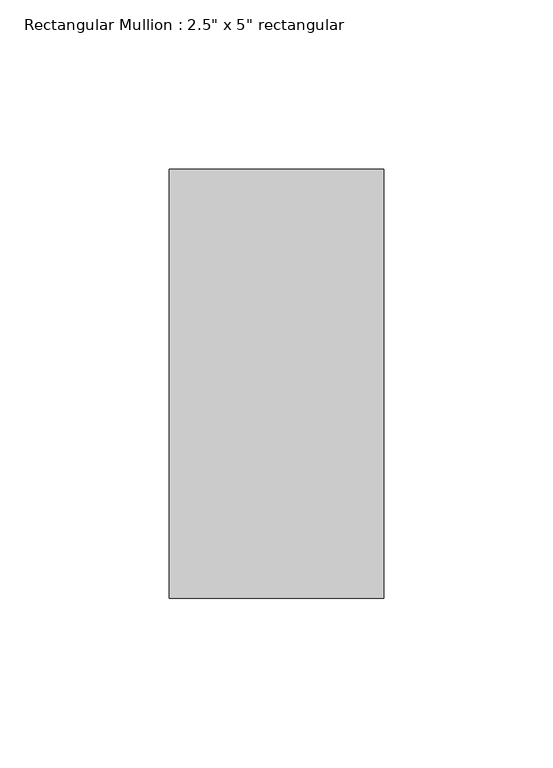
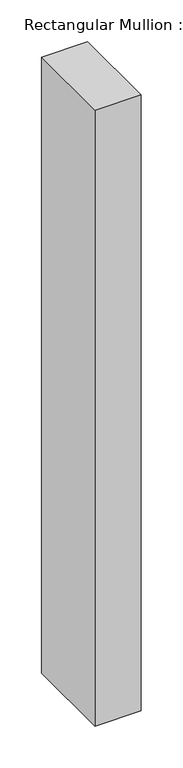
"""IFC4 building model written with IfcOpenShell, lengths in millimetres: member geometry."""

from ifc_helpers import new_model, si_unit, frame, origin, place, context, project, spatial, polyline, outline, extrude, source, transform, mapped, element, save


def member_9cc26bde(model_context):
    return source(origin(), model_context, "Body", "SweptSolid", [
        extrude(outline(polyline([(31.75, 63.5), (31.75, -63.5), (-31.75, -63.5), (-31.75, 63.5), (31.75, 63.5)])), frame((0.0, 0.0, -897.4039078), z_axis=(0.0, 0.0, 1.0), x_axis=(1.0, 0.0, 0.0)), (0.0, 0.0, 1.0), 897.4039078),
    ])


if __name__ == "__main__":
    model = new_model("IFC4")
    model_context = context("Model", 3, world=origin())
    ifc_project = project(units=[si_unit("LENGTHUNIT", "METRE", prefix="MILLI")], contexts=[model_context])
    site = spatial("IfcSite", under=ifc_project)
    building = spatial("IfcBuilding", under=site)
    placement = place(None, origin())
    member_shape = member_9cc26bde(model_context)
    element("IfcMember", 1, ObjectType="Rectangular Mullion : 2.5\" x 5\" rectangular", at=placement, inside=building, context=model_context, shape_type="MappedRepresentation", body=[
        mapped(member_shape, transform((0.0, 0.0, 0.0), x_axis=(1.0, 0.0, 0.0), y_axis=(0.0, 1.0, 0.0), z_axis=(0.0, 0.0, 1.0))),
    ])
    save(model, "model.ifc")

# Revit data of these elements
# Type "Rectangular Mullion : 2.5\" x 5\" rectangular"
#   built-in parameter 1007304 = 0.416667 (stored number, unit not read)
#   built-in parameter 1007301 = 0.104167 (stored number, unit not read)
#   built-in parameter 1007300 = 0.104167 (stored number, unit not read)
# Element 1 (IfcMember, "Rectangular Mullion : 2.5\" x 5\" rectangular")
#   Materials on its faces: "Aluminum"
# Materials
#   "Aluminum": class "Metal", colour RGB 247 247 247, transparency 0, Description = "Aluminum 6061", Cost = 0
